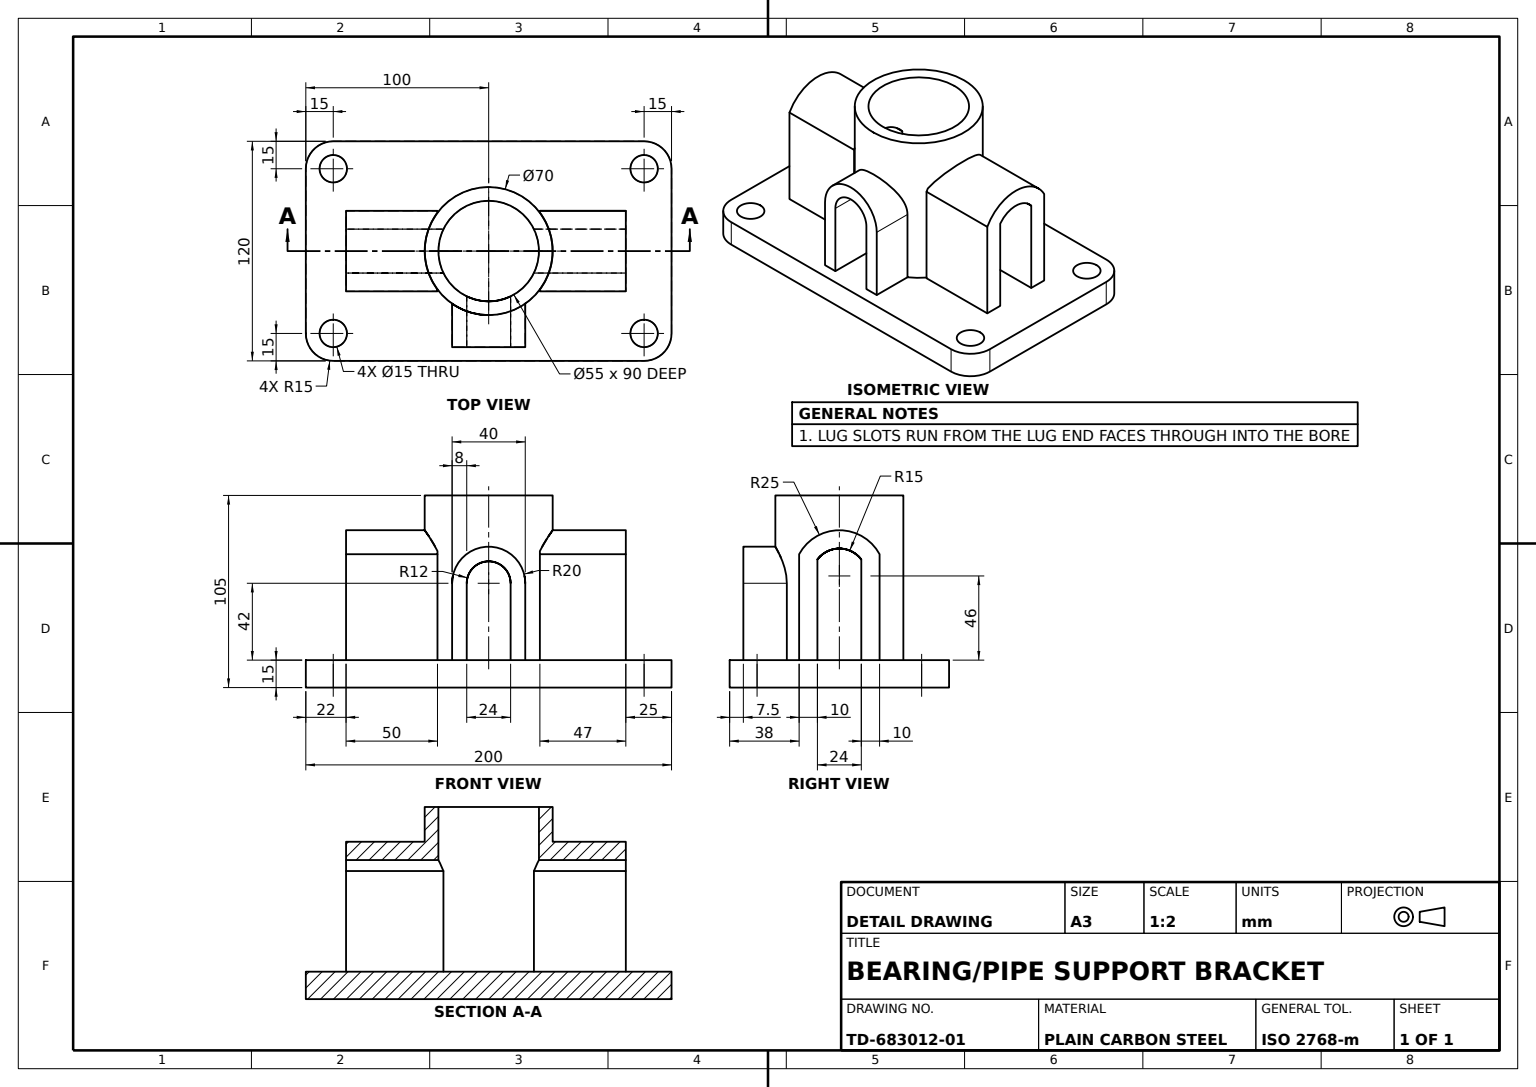
from build123d import *

# Parameters (mm, degrees)
BASE_PLATE_SKETCH_R         = 7.5
BASE_PLATE_200X120X15_DEPTH = 15
TUBE_BOSS_SKETCH_R          = 35
TUBE_BOSS_SKETCH_R_2        = 27.5
TUBE_BOSS_55_BORE_35_DEPTH  = 90
FRONT_LUG_DEPTH             = 24
FRONT_LUG_CUT_DEPTH         = 40
SIDE_LUG_A_DEPTH            = 3
SIDE_LUG_A_DEPTH_BACK       = 47
SIDE_START                  = -73
SIDE_LUG_A_SLOT_DEPTH       = 73
SIDE_LUG_B_DEPTH            = 47
SIDE_LUG_B_SLOT_DEPTH       = 67


with BuildPart() as part:
    # Base Plate Sketch → Base Plate 200x120x15 (new body)
    with BuildSketch(Plane(origin=(0, 0, 0), x_dir=(1, 0, 0), z_dir=(0, 1, 0))):
        with BuildLine():
            Line((-85, -60), (85, -60))
            ThreePointArc((85, -60), (95.606601718, -55.606601718), (100, -45))
            Line((100, -45), (100, 45))
            ThreePointArc((100, 45), (95.606601718, 55.606601718), (85, 60))
            Line((85, 60), (-85, 60))
            ThreePointArc((-85, 60), (-95.606601718, 55.606601718), (-100, 45))
            Line((-100, 45), (-100, -45))
            ThreePointArc((-100, -45), (-95.606601718, -55.606601718), (-85, -60))
        make_face()
        with Locations(Location((-85, 45, 0), (0, 0, 270))):
            Circle(BASE_PLATE_SKETCH_R, mode=Mode.SUBTRACT)
        with Locations(Location((85, 45, 0), (0, 0, 270))):
            Circle(BASE_PLATE_SKETCH_R, mode=Mode.SUBTRACT)
        with Locations(Location((85, -45, 0), (0, 0, 270))):
            Circle(BASE_PLATE_SKETCH_R, mode=Mode.SUBTRACT)
        with Locations(Location((-85, -45, 0), (0, 0, 270))):
            Circle(BASE_PLATE_SKETCH_R, mode=Mode.SUBTRACT)
    extrude(amount=BASE_PLATE_200X120X15_DEPTH)

    # Tube Boss Sketch → Tube Boss Ø55 Bore Ø35 (add)
    with BuildSketch(Plane(origin=(0, 15, 0), x_dir=(1, 0, 0), z_dir=(0, 1, 0))):
        with Locations(Location((0, 0, 0), (0, 0, 90))):
            Circle(TUBE_BOSS_SKETCH_R)
        with Locations(Location((0, 0, 0), (0, 0, 90))):
            Circle(TUBE_BOSS_SKETCH_R_2, mode=Mode.SUBTRACT)
    extrude(amount=TUBE_BOSS_55_BORE_35_DEPTH)

    # Front Lug Sketch → Front Lug (add)
    with BuildSketch(Plane.XY.offset(52.5)):
        with BuildLine():
            Line((-12, 15), (-12, 57))
            ThreePointArc((-12, 57), (0, 69), (12, 57))
            Line((12, 57), (12, 15))
            Line((12, 15), (20, 15))
            Line((20, 15), (20, 57))
            ThreePointArc((20, 57), (0, 77), (-20, 57))
            Line((-20, 57), (-20, 15))
            Line((-20, 15), (-12, 15))
        make_face()
    extrude(amount=-FRONT_LUG_DEPTH)

    # Front Lug Cut Sketch → Front Lug Cut (cut)
    with BuildSketch(Plane.XY.offset(52.5)):
        with BuildLine():
            Line((-12, 15), (12, 15))
            Line((12, 15), (12, 57))
            ThreePointArc((12, 57), (0, 69), (-12, 57))
            Line((-12, 57), (-12, 15))
        make_face()
    extrude(amount=-FRONT_LUG_CUT_DEPTH, mode=Mode.SUBTRACT)

    # Side Lug A Sketch → Side Lug A (add, two sides: drawn at the far end of the back side and taken through both)
    with BuildSketch(Plane.ZY.offset(75).offset(-SIDE_LUG_A_DEPTH_BACK)):
        with BuildLine():
            Line((-12, 15), (-12, 70))
            ThreePointArc((-12, 70), (0, 76), (12, 70))
            Line((12, 70), (12, 15))
            Line((12, 15), (22, 15))
            Line((22, 15), (22, 72.874342087))
            ThreePointArc((22, 72.874342087), (0, 86), (-22, 72.874342087))
            Line((-22, 72.874342087), (-22, 15))
            Line((-22, 15), (-12, 15))
        make_face()
    extrude(amount=SIDE_LUG_A_DEPTH + SIDE_LUG_A_DEPTH_BACK)

    # Side Lug A Slot Sketch → Side Lug A Slot (cut)
    with BuildSketch(Plane.ZY.offset(78).offset(SIDE_START)):
        with BuildLine():
            Line((12, 70), (12, 15))
            Line((12, 15), (-12, 15))
            Line((-12, 15), (-12, 70))
            ThreePointArc((-12, 70), (0, 76), (12, 70))
        make_face()
    extrude(amount=SIDE_LUG_A_SLOT_DEPTH, mode=Mode.SUBTRACT)

    # Side Lug B Sketch → Side Lug B (add)
    with BuildSketch(Plane(origin=(75, 0, 0), x_dir=(0, 0, -1), z_dir=(1, 0, 0))):
        with BuildLine():
            Line((-12, 15), (-12, 70))
            ThreePointArc((-12, 70), (0, 76), (12, 70))
            Line((12, 70), (12, 15))
            Line((12, 15), (22, 15))
            Line((22, 15), (22, 72.874342087))
            ThreePointArc((22, 72.874342087), (0, 86), (-22, 72.874342087))
            Line((-22, 72.874342087), (-22, 15))
            Line((-22, 15), (-12, 15))
        make_face()
    extrude(amount=-SIDE_LUG_B_DEPTH)

    # Side Lug B Slot Sketch → Side Lug B Slot (cut)
    with BuildSketch(Plane(origin=(75, 0, 0), x_dir=(0, 0, -1), z_dir=(1, 0, 0))):
        with BuildLine():
            Line((12, 15), (12, 70))
            ThreePointArc((12, 70), (0, 76), (-12, 70))
            Line((-12, 70), (-12, 15))
            Line((-12, 15), (12, 15))
        make_face()
    extrude(amount=-SIDE_LUG_B_SLOT_DEPTH, mode=Mode.SUBTRACT)


solid = part.part
